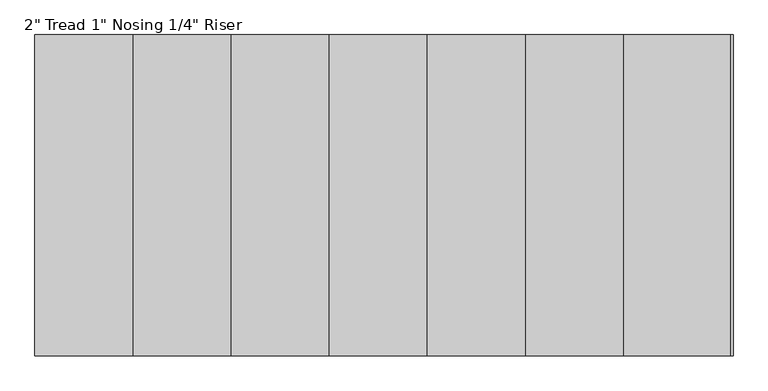
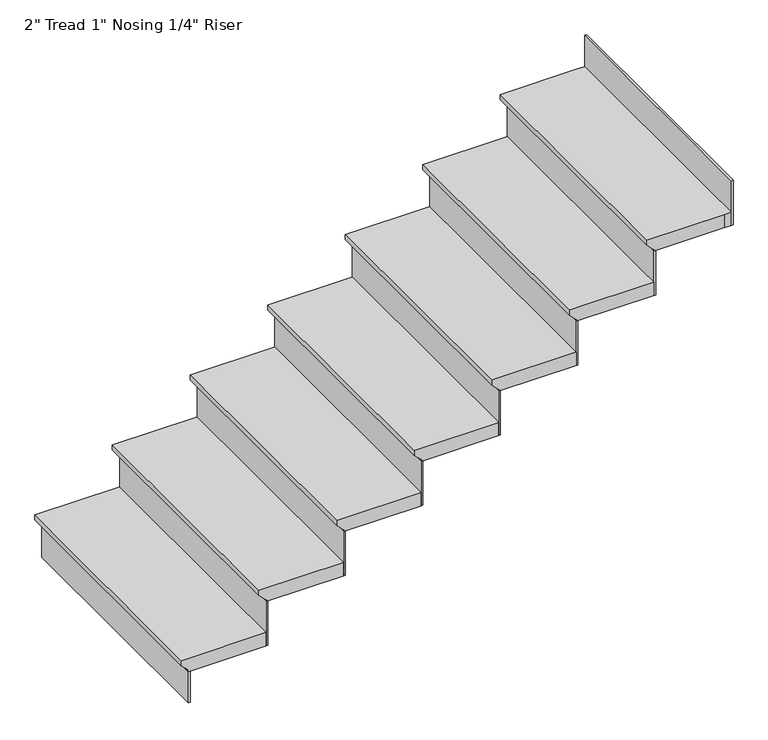
"""IFC4 building model written with IfcOpenShell, lengths in millimetres: stair flight geometry."""

from ifc_helpers import new_model, si_unit, origin, place, context, project, spatial, faceted_brep, source, transform, mapped, element, save


def stair_flight_33a07897(model_context):
    return source(origin(), model_context, "Body", "Brep", [
        faceted_brep([(-1552.2130387, 2354.550634, 9903.8833333), (-1552.2130387, 2354.550634, 9922.9333333), (-1552.2130387, 3268.950634, 9922.9333333), (-1552.2130387, 3268.950634, 9903.8833333), (-1526.8130387, 2354.550634, 9878.4833333), (-1526.8130387, 3268.950634, 9878.4833333), (-1247.4130387, 2354.550634, 9922.9333333), (-1247.4130387, 3268.950634, 9922.9333333), (-1526.8130387, 3268.950634, 9872.1333333), (-1247.4130387, 3268.950634, 9872.1333333), (-1247.4130387, 2354.550634, 9872.1333333), (-1526.8130387, 2354.550634, 9872.1333333)], [[[0, 1, 2, 3]], [[4, 0, 3, 5]], [[2, 1, 6, 7]], [[8, 9, 10, 11]], [[2, 7, 9, 8, 5, 3]], [[8, 11, 4, 5]], [[6, 1, 0, 4, 11, 10]], [[7, 6, 10, 9]]]),
        faceted_brep([(-1526.8130387, 2354.550634, 9872.1333333), (-1526.8130387, 2354.550634, 9753.6), (-1520.4630387, 2354.550634, 9753.6), (-1520.4630387, 2354.550634, 9872.1333333), (-1526.8130387, 3268.950634, 9872.1333333), (-1520.4630387, 3268.950634, 9872.1333333), (-1520.4630387, 3268.950634, 9753.6), (-1526.8130387, 3268.950634, 9753.6)], [[[0, 1, 2, 3]], [[4, 5, 6, 7]], [[1, 0, 4, 7]], [[2, 1, 7, 6]], [[3, 2, 6, 5]], [[0, 3, 5, 4]]]),
        faceted_brep([(-1247.4130387, 2354.550634, 10041.4666667), (-1247.4130387, 2354.550634, 9872.1333333), (-1241.0630387, 2354.550634, 9872.1333333), (-1241.0630387, 2354.550634, 10041.4666667), (-1247.4130387, 3268.950634, 10041.4666667), (-1241.0630387, 3268.950634, 10041.4666667), (-1241.0630387, 3268.950634, 9872.1333333), (-1247.4130387, 3268.950634, 9872.1333333)], [[[0, 1, 2, 3]], [[4, 5, 6, 7]], [[1, 0, 4, 7]], [[2, 1, 7, 6]], [[3, 2, 6, 5]], [[0, 3, 5, 4]]]),
        faceted_brep([(-1272.8130387, 3268.950634, 10092.2666667), (-1272.8130387, 2354.550634, 10092.2666667), (-968.0130387, 2354.550634, 10092.2666667), (-968.0130387, 3268.950634, 10092.2666667), (-1247.4130387, 3268.950634, 10041.4666667), (-968.0130387, 3268.950634, 10041.4666667), (-968.0130387, 2354.550634, 10041.4666667), (-1247.4130387, 2354.550634, 10041.4666667), (-1247.4130387, 3268.950634, 10047.8166667), (-1272.8130387, 3268.950634, 10073.2166667), (-1247.4130387, 2354.550634, 10047.8166667), (-1272.8130387, 2354.550634, 10073.2166667)], [[[0, 1, 2, 3]], [[4, 5, 6, 7]], [[0, 3, 5, 4, 8, 9]], [[4, 7, 10, 8]], [[2, 1, 11, 10, 7, 6]], [[3, 2, 6, 5]], [[11, 1, 0, 9]], [[10, 11, 9, 8]]]),
        faceted_brep([(-968.0130387, 2354.550634, 10210.8), (-968.0130387, 2354.550634, 10041.4666667), (-961.6630387, 2354.550634, 10041.4666667), (-961.6630387, 2354.550634, 10210.8), (-968.0130387, 3268.950634, 10210.8), (-961.6630387, 3268.950634, 10210.8), (-961.6630387, 3268.950634, 10041.4666667), (-968.0130387, 3268.950634, 10041.4666667)], [[[0, 1, 2, 3]], [[4, 5, 6, 7]], [[1, 0, 4, 7]], [[2, 1, 7, 6]], [[3, 2, 6, 5]], [[0, 3, 5, 4]]]),
        faceted_brep([(-993.4130387, 3268.950634, 10261.6), (-993.4130387, 2354.550634, 10261.6), (-688.6130387, 2354.550634, 10261.6), (-688.6130387, 3268.950634, 10261.6), (-968.0130387, 3268.950634, 10210.8), (-688.6130387, 3268.950634, 10210.8), (-688.6130387, 2354.550634, 10210.8), (-968.0130387, 2354.550634, 10210.8), (-968.0130387, 3268.950634, 10217.15), (-993.4130387, 3268.950634, 10242.55), (-968.0130387, 2354.550634, 10217.15), (-993.4130387, 2354.550634, 10242.55)], [[[0, 1, 2, 3]], [[4, 5, 6, 7]], [[0, 3, 5, 4, 8, 9]], [[4, 7, 10, 8]], [[2, 1, 11, 10, 7, 6]], [[3, 2, 6, 5]], [[11, 1, 0, 9]], [[10, 11, 9, 8]]]),
        faceted_brep([(-688.6130387, 2354.550634, 10380.1333333), (-688.6130387, 2354.550634, 10210.8), (-682.2630387, 2354.550634, 10210.8), (-682.2630387, 2354.550634, 10380.1333333), (-688.6130387, 3268.950634, 10380.1333333), (-682.2630387, 3268.950634, 10380.1333333), (-682.2630387, 3268.950634, 10210.8), (-688.6130387, 3268.950634, 10210.8)], [[[0, 1, 2, 3]], [[4, 5, 6, 7]], [[1, 0, 4, 7]], [[2, 1, 7, 6]], [[3, 2, 6, 5]], [[0, 3, 5, 4]]]),
        faceted_brep([(-714.0130387, 3268.950634, 10430.9333333), (-714.0130387, 2354.550634, 10430.9333333), (-409.2130387, 2354.550634, 10430.9333333), (-409.2130387, 3268.950634, 10430.9333333), (-688.6130387, 3268.950634, 10380.1333333), (-409.2130387, 3268.950634, 10380.1333333), (-409.2130387, 2354.550634, 10380.1333333), (-688.6130387, 2354.550634, 10380.1333333), (-688.6130387, 3268.950634, 10386.4833333), (-714.0130387, 3268.950634, 10411.8833333), (-688.6130387, 2354.550634, 10386.4833333), (-714.0130387, 2354.550634, 10411.8833333)], [[[0, 1, 2, 3]], [[4, 5, 6, 7]], [[0, 3, 5, 4, 8, 9]], [[4, 7, 10, 8]], [[2, 1, 11, 10, 7, 6]], [[3, 2, 6, 5]], [[11, 1, 0, 9]], [[10, 11, 9, 8]]]),
        faceted_brep([(-409.2130387, 2354.550634, 10549.4666667), (-409.2130387, 2354.550634, 10380.1333333), (-402.8630387, 2354.550634, 10380.1333333), (-402.8630387, 2354.550634, 10549.4666667), (-409.2130387, 3268.950634, 10549.4666667), (-402.8630387, 3268.950634, 10549.4666667), (-402.8630387, 3268.950634, 10380.1333333), (-409.2130387, 3268.950634, 10380.1333333)], [[[0, 1, 2, 3]], [[4, 5, 6, 7]], [[1, 0, 4, 7]], [[2, 1, 7, 6]], [[3, 2, 6, 5]], [[0, 3, 5, 4]]]),
        faceted_brep([(-434.6130387, 3268.950634, 10600.2666667), (-434.6130387, 2354.550634, 10600.2666667), (-129.8130387, 2354.550634, 10600.2666667), (-129.8130387, 3268.950634, 10600.2666667), (-409.2130387, 3268.950634, 10549.4666667), (-129.8130387, 3268.950634, 10549.4666667), (-129.8130387, 2354.550634, 10549.4666667), (-409.2130387, 2354.550634, 10549.4666667), (-409.2130387, 3268.950634, 10555.8166667), (-434.6130387, 3268.950634, 10581.2166667), (-409.2130387, 2354.550634, 10555.8166667), (-434.6130387, 2354.550634, 10581.2166667)], [[[0, 1, 2, 3]], [[4, 5, 6, 7]], [[0, 3, 5, 4, 8, 9]], [[4, 7, 10, 8]], [[2, 1, 11, 10, 7, 6]], [[3, 2, 6, 5]], [[11, 1, 0, 9]], [[10, 11, 9, 8]]]),
        faceted_brep([(-129.8130387, 2354.550634, 10718.8), (-129.8130387, 2354.550634, 10549.4666667), (-123.4630387, 2354.550634, 10549.4666667), (-123.4630387, 2354.550634, 10718.8), (-129.8130387, 3268.950634, 10718.8), (-123.4630387, 3268.950634, 10718.8), (-123.4630387, 3268.950634, 10549.4666667), (-129.8130387, 3268.950634, 10549.4666667)], [[[0, 1, 2, 3]], [[4, 5, 6, 7]], [[1, 0, 4, 7]], [[2, 1, 7, 6]], [[3, 2, 6, 5]], [[0, 3, 5, 4]]]),
        faceted_brep([(-155.2130387, 3268.950634, 10769.6), (-155.2130387, 2354.550634, 10769.6), (149.5869613, 2354.550634, 10769.6), (149.5869613, 3268.950634, 10769.6), (-129.8130387, 3268.950634, 10718.8), (149.5869613, 3268.950634, 10718.8), (149.5869613, 2354.550634, 10718.8), (-129.8130387, 2354.550634, 10718.8), (-129.8130387, 3268.950634, 10725.15), (-155.2130387, 3268.950634, 10750.55), (-129.8130387, 2354.550634, 10725.15), (-155.2130387, 2354.550634, 10750.55)], [[[0, 1, 2, 3]], [[4, 5, 6, 7]], [[0, 3, 5, 4, 8, 9]], [[4, 7, 10, 8]], [[2, 1, 11, 10, 7, 6]], [[3, 2, 6, 5]], [[11, 1, 0, 9]], [[10, 11, 9, 8]]]),
        faceted_brep([(428.9869613, 2354.550634, 11057.4666667), (428.9869613, 2354.550634, 10888.1333333), (435.3369613, 2354.550634, 10888.1333333), (435.3369613, 2354.550634, 11057.4666667), (428.9869613, 3268.950634, 11057.4666667), (435.3369613, 3268.950634, 11057.4666667), (435.3369613, 3268.950634, 10888.1333333), (428.9869613, 3268.950634, 10888.1333333)], [[[0, 1, 2, 3]], [[4, 5, 6, 7]], [[1, 0, 4, 7]], [[2, 1, 7, 6]], [[3, 2, 6, 5]], [[0, 3, 5, 4]]]),
        faceted_brep([(149.5869613, 2354.550634, 10888.1333333), (149.5869613, 2354.550634, 10718.8), (155.9369613, 2354.550634, 10718.8), (155.9369613, 2354.550634, 10888.1333333), (149.5869613, 3268.950634, 10888.1333333), (155.9369613, 3268.950634, 10888.1333333), (155.9369613, 3268.950634, 10718.8), (149.5869613, 3268.950634, 10718.8)], [[[0, 1, 2, 3]], [[4, 5, 6, 7]], [[1, 0, 4, 7]], [[2, 1, 7, 6]], [[3, 2, 6, 5]], [[0, 3, 5, 4]]]),
        faceted_brep([(428.9869613, 3268.950634, 10938.9333333), (403.5869613, 3268.950634, 10938.9333333), (124.1869613, 3268.950634, 10938.9333333), (124.1869613, 2354.550634, 10938.9333333), (403.5869613, 2354.550634, 10938.9333333), (428.9869613, 2354.550634, 10938.9333333), (403.5869613, 3268.950634, 10888.1333333), (428.9869613, 3268.950634, 10888.1333333), (428.9869613, 2354.550634, 10888.1333333), (403.5869613, 2354.550634, 10888.1333333), (149.5869613, 2354.550634, 10888.1333333), (149.5869613, 3268.950634, 10888.1333333), (149.5869613, 3268.950634, 10894.4833333), (124.1869613, 3268.950634, 10919.8833333), (149.5869613, 2354.550634, 10894.4833333), (124.1869613, 2354.550634, 10919.8833333)], [[[0, 1, 2, 3, 4, 5]], [[6, 7, 8, 9, 10, 11]], [[1, 0, 7, 6]], [[2, 1, 6, 11, 12, 13]], [[11, 10, 14, 12]], [[4, 3, 15, 14, 10, 9]], [[5, 4, 9, 8]], [[0, 5, 8, 7]], [[15, 3, 2, 13]], [[14, 15, 13, 12]]]),
    ])


if __name__ == "__main__":
    model = new_model("IFC4")
    model_context = context("Model", 3, world=origin())
    ifc_project = project(units=[si_unit("LENGTHUNIT", "METRE", prefix="MILLI")], contexts=[model_context])
    site = spatial("IfcSite", under=ifc_project)
    building = spatial("IfcBuilding", under=site)
    placement = place(None, origin())
    stair_flight_shape = stair_flight_33a07897(model_context)
    element("IfcStairFlight", 1, ObjectType="2\" Tread 1\" Nosing 1/4\" Riser", at=placement, inside=building, context=model_context, shape_type="MappedRepresentation", body=[
        mapped(stair_flight_shape, transform((0.0, 0.0, 0.0), x_axis=(1.0, 0.0, 0.0), y_axis=(0.0, 1.0, 0.0), z_axis=(0.0, 0.0, 1.0))),
    ])
    save(model, "model.ifc")

# Revit data of these elements
# Element 1 (IfcStairFlight, "2\" Tread 1\" Nosing 1/4\" Riser")
#   Materials on its faces: "BURGUNDY COLOUR"
# Materials
#   "BURGUNDY COLOUR": class "Generic", colour RGB 120 120 120, transparency 0, Cost = 0
